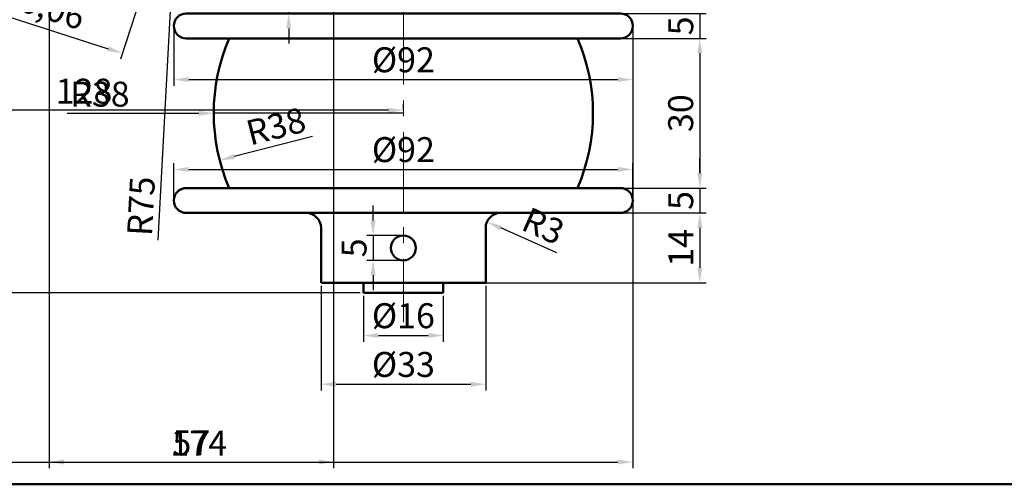
# Model space of a CAD drawing. Units: millimetres. Extents: x 98 to 674, y 38 to 476.
# Tile 2 of 7: x 200 to 398, y 38 to 131. Entities that reach past the tile are written whole.
import ezdxf

# ---------------------------------------------------------------- set-up
doc = ezdxf.new("R2010")
doc.units = ezdxf.units.MM
doc.header["$LTSCALE"] = 0.5
doc.linetypes.add('CENTER', pattern=[50.8, 31.75, -6.35, 6.35, -6.35])
for name, color, linetype, lineweight in [('M-CNTR', 1, 'CENTER', 18), ('M-DIMS', 2, 'Continuous', 25), ('M-OUTL', 7, 'Continuous', 50), ('M-TTLB', 7, 'Continuous', 50)]:
    doc.layers.add(name, color=color, linetype=linetype, lineweight=lineweight)
doc.styles.get("Standard").update_dxf_attribs({"font": 'arial.ttf'})
doc.dimstyles.new('ISO-25', dxfattribs={"dimtxt": 5, "dimasz": 3, "dimexe": 1.25, "dimexo": 0.625, "dimtad": 1, "dimtxsty": 'Standard', "dimcen": 2.5, "dimadec": 0, "dimazin": 0, "dimtfac": 1, "dimtmove": 0, "dimatfit": 3, "dimfxl": 1, "dimarcsym": 0})

# ---------------------------------------------------------------- blocks, each defined once
blk = doc.blocks.new('*D38')
at = {"layer": 'Defpoints', "color": 0, "ltscale": 0.5, "transparency": 16777216}
for p in [(254.39, 138.69), (254.39, 132.69), (254.39, 132.69)]:
    blk.add_point(p, dxfattribs=at)
at = {"layer": 'M-DIMS', "color": 0, "lineweight": -2, "ltscale": 0.5, "transparency": 16777216}
for p, q in [((254.39, 141.69), (254.39, 144.69)), ((254.39, 138.69), (254.39, 132.69)), ((255.02, 138.69), (255.64, 138.69)), ((255.02, 132.69), (255.64, 132.69)), ((254.39, 129.69), (254.39, 126.69))]:
    blk.add_line(p, q, dxfattribs=at)
at = {"layer": 'M-DIMS', "color": 0, "ltscale": 0.5, "transparency": 16777216}
for points in [[(253.89, 141.69), (254.89, 141.69), (254.39, 138.69)], [(253.89, 129.69), (254.89, 129.69), (254.39, 132.69)]]:
    blk.add_solid(points, dxfattribs=at)
at = {"layer": 'M-DIMS', "color": 0, "ltscale": 0.5, "transparency": 16777216, "insert": (251.21, 135.69), "char_height": 5, "attachment_point": 5, "rotation": 90}
blk.add_mtext('6', dxfattribs=at)
blk = doc.blocks.new('*D39')
at = {"layer": 'Defpoints', "color": 0, "ltscale": 0.5, "transparency": 16777216}
for p in [(231.37, 130.19), (323.37, 130.19), (323.37, 119.43)]:
    blk.add_point(p, dxfattribs=at)
at = {"layer": 'M-DIMS', "color": 0, "lineweight": -2, "ltscale": 0.5, "transparency": 16777216}
for p, q in [((231.37, 129.56), (231.37, 118.18)), ((323.37, 129.56), (323.37, 118.18)), ((234.37, 119.43), (320.37, 119.43))]:
    blk.add_line(p, q, dxfattribs=at)
at = {"layer": 'M-DIMS', "color": 0, "ltscale": 0.5, "transparency": 16777216}
for points in [[(234.37, 119.93), (234.37, 118.93), (231.37, 119.43)], [(320.37, 119.93), (320.37, 118.93), (323.37, 119.43)]]:
    blk.add_solid(points, dxfattribs=at)
at = {"layer": 'M-DIMS', "color": 0, "ltscale": 0.5, "transparency": 16777216, "insert": (277.37, 122.75), "char_height": 5, "attachment_point": 5}
blk.add_mtext('%%C92', dxfattribs=at)
blk = doc.blocks.new('*D40')
at = {"layer": 'Defpoints', "color": 0, "ltscale": 0.5, "transparency": 16777216}
for p in [(277.37, 112.69), (240.56, 103.24)]:
    blk.add_point(p, dxfattribs=at)
at = {"layer": 'M-DIMS', "color": 0, "lineweight": -2, "ltscale": 0.5, "transparency": 16777216}
blk.add_line((259.16, 108.02), (243.46, 103.99), dxfattribs=at)
at = {"layer": 'M-DIMS', "color": 0, "ltscale": 0.5, "transparency": 16777216}
blk.add_solid([(243.34, 104.47), (243.59, 103.5), (240.56, 103.24)], dxfattribs=at)
at = {"layer": 'M-DIMS', "color": 0, "ltscale": 0.5, "transparency": 16777216, "insert": (251.98, 109.45), "char_height": 5, "attachment_point": 5, "rotation": 14.3875}
blk.add_mtext('R38', dxfattribs=at)
blk = doc.blocks.new('*D41')
at = {"layer": 'Defpoints', "color": 0, "ltscale": 0.5, "transparency": 16777216}
for p in [(323.37, 101.42), (231.37, 95.19), (323.37, 95.19)]:
    blk.add_point(p, dxfattribs=at)
at = {"layer": 'M-DIMS', "color": 0, "lineweight": -2, "ltscale": 0.5, "transparency": 16777216}
for p, q in [((231.37, 95.81), (231.37, 102.67)), ((323.37, 95.81), (323.37, 102.67)), ((234.37, 101.42), (320.37, 101.42))]:
    blk.add_line(p, q, dxfattribs=at)
at = {"layer": 'M-DIMS', "color": 0, "ltscale": 0.5, "transparency": 16777216}
for points in [[(234.37, 101.92), (234.37, 100.92), (231.37, 101.42)], [(320.37, 101.92), (320.37, 100.92), (323.37, 101.42)]]:
    blk.add_solid(points, dxfattribs=at)
at = {"layer": 'M-DIMS', "color": 0, "ltscale": 0.5, "transparency": 16777216, "insert": (277.37, 104.74), "char_height": 5, "attachment_point": 5}
blk.add_mtext('%%C92', dxfattribs=at)
blk = doc.blocks.new('*D42')
at = {"layer": 'Defpoints', "color": 0, "ltscale": 0.5, "transparency": 16777216}
for p in [(316.66, 132.69), (316.66, 127.69), (336.77, 127.69)]:
    blk.add_point(p, dxfattribs=at)
at = {"layer": 'M-DIMS', "color": 0, "lineweight": -2, "ltscale": 0.5, "transparency": 16777216}
for p, q in [((336.77, 135.69), (336.77, 138.69)), ((317.29, 132.69), (338.02, 132.69)), ((336.77, 132.69), (336.77, 127.69)), ((317.29, 127.69), (338.02, 127.69)), ((336.77, 124.69), (336.77, 121.69))]:
    blk.add_line(p, q, dxfattribs=at)
at = {"layer": 'M-DIMS', "color": 0, "ltscale": 0.5, "transparency": 16777216}
for points in [[(336.27, 135.69), (337.27, 135.69), (336.77, 132.69)], [(336.27, 124.69), (337.27, 124.69), (336.77, 127.69)]]:
    blk.add_solid(points, dxfattribs=at)
at = {"layer": 'M-DIMS', "color": 0, "ltscale": 0.5, "transparency": 16777216, "insert": (333.6, 130.19), "char_height": 5, "attachment_point": 5, "rotation": 90}
blk.add_mtext('5', dxfattribs=at)
blk = doc.blocks.new('*D43')
at = {"layer": 'Defpoints', "color": 0, "ltscale": 0.5, "transparency": 16777216}
for p in [(316.66, 127.69), (316.66, 97.69), (336.77, 97.69)]:
    blk.add_point(p, dxfattribs=at)
at = {"layer": 'M-DIMS', "color": 0, "lineweight": -2, "ltscale": 0.5, "transparency": 16777216}
for p, q in [((317.29, 127.69), (338.02, 127.69)), ((336.77, 124.69), (336.77, 100.69)), ((317.29, 97.69), (338.02, 97.69))]:
    blk.add_line(p, q, dxfattribs=at)
at = {"layer": 'M-DIMS', "color": 0, "ltscale": 0.5, "transparency": 16777216}
for points in [[(336.27, 124.69), (337.27, 124.69), (336.77, 127.69)], [(336.27, 100.69), (337.27, 100.69), (336.77, 97.69)]]:
    blk.add_solid(points, dxfattribs=at)
at = {"layer": 'M-DIMS', "color": 0, "ltscale": 0.5, "transparency": 16777216, "insert": (333.59, 112.69), "char_height": 5, "attachment_point": 5, "rotation": 90}
blk.add_mtext('30', dxfattribs=at)
blk = doc.blocks.new('*D44')
at = {"layer": 'Defpoints', "color": 0, "ltscale": 0.5, "transparency": 16777216}
for p in [(316.66, 97.69), (316.66, 92.69), (336.77, 92.69)]:
    blk.add_point(p, dxfattribs=at)
at = {"layer": 'M-DIMS', "color": 0, "lineweight": -2, "ltscale": 0.5, "transparency": 16777216}
for p, q in [((336.77, 100.69), (336.77, 103.69)), ((317.29, 97.69), (338.02, 97.69)), ((336.77, 97.69), (336.77, 92.69)), ((317.29, 92.69), (338.02, 92.69)), ((336.77, 89.69), (336.77, 86.69))]:
    blk.add_line(p, q, dxfattribs=at)
at = {"layer": 'M-DIMS', "color": 0, "ltscale": 0.5, "transparency": 16777216}
for points in [[(336.27, 100.69), (337.27, 100.69), (336.77, 97.69)], [(336.27, 89.69), (337.27, 89.69), (336.77, 92.69)]]:
    blk.add_solid(points, dxfattribs=at)
at = {"layer": 'M-DIMS', "color": 0, "ltscale": 0.5, "transparency": 16777216, "insert": (333.6, 95.19), "char_height": 5, "attachment_point": 5, "rotation": 90}
blk.add_mtext('5', dxfattribs=at)
blk = doc.blocks.new('*D45')
at = {"layer": 'Defpoints', "color": 0, "ltscale": 0.5, "transparency": 16777216}
for p in [(288.74, 92.69), (288.74, 78.69), (336.77, 78.69)]:
    blk.add_point(p, dxfattribs=at)
at = {"layer": 'M-DIMS', "color": 0, "lineweight": -2, "ltscale": 0.5, "transparency": 16777216}
for p, q in [((289.36, 92.69), (338.02, 92.69)), ((336.77, 89.69), (336.77, 81.69)), ((289.36, 78.69), (338.02, 78.69))]:
    blk.add_line(p, q, dxfattribs=at)
at = {"layer": 'M-DIMS', "color": 0, "ltscale": 0.5, "transparency": 16777216}
for points in [[(336.27, 89.69), (337.27, 89.69), (336.77, 92.69)], [(336.27, 81.69), (337.27, 81.69), (336.77, 78.69)]]:
    blk.add_solid(points, dxfattribs=at)
at = {"layer": 'M-DIMS', "color": 0, "ltscale": 0.5, "transparency": 16777216, "insert": (333.64, 85.69), "char_height": 5, "attachment_point": 5, "rotation": 90}
blk.add_mtext('14', dxfattribs=at)
blk = doc.blocks.new('*D46')
at = {"layer": 'Defpoints', "color": 0, "ltscale": 0.5, "transparency": 16777216}
for p in [(277.37, 88.19), (271.3, 83.19), (277.37, 83.19)]:
    blk.add_point(p, dxfattribs=at)
at = {"layer": 'M-DIMS', "color": 0, "lineweight": -2, "ltscale": 0.5, "transparency": 16777216}
for p, q in [((271.3, 91.19), (271.3, 94.19)), ((276.74, 88.19), (270.05, 88.19)), ((271.3, 88.19), (271.3, 83.19)), ((276.74, 83.19), (270.05, 83.19)), ((271.3, 80.19), (271.3, 77.19))]:
    blk.add_line(p, q, dxfattribs=at)
at = {"layer": 'M-DIMS', "color": 0, "ltscale": 0.5, "transparency": 16777216}
for points in [[(270.8, 91.19), (271.8, 91.19), (271.3, 88.19)], [(270.8, 80.19), (271.8, 80.19), (271.3, 83.19)]]:
    blk.add_solid(points, dxfattribs=at)
at = {"layer": 'M-DIMS', "color": 0, "ltscale": 0.5, "transparency": 16777216, "insert": (268.13, 85.69), "char_height": 5, "attachment_point": 5, "rotation": 90}
blk.add_mtext('5', dxfattribs=at)
blk = doc.blocks.new('*D47')
at = {"layer": 'Defpoints', "color": 0, "ltscale": 0.5, "transparency": 16777216}
for p in [(269.37, 76.69), (285.37, 76.69), (285.37, 68.12)]:
    blk.add_point(p, dxfattribs=at)
at = {"layer": 'M-DIMS', "color": 0, "lineweight": -2, "ltscale": 0.5, "transparency": 16777216}
for p, q in [((269.37, 76.06), (269.37, 66.87)), ((285.37, 76.06), (285.37, 66.87)), ((272.37, 68.12), (282.37, 68.12))]:
    blk.add_line(p, q, dxfattribs=at)
at = {"layer": 'M-DIMS', "color": 0, "ltscale": 0.5, "transparency": 16777216}
for points in [[(272.37, 68.62), (272.37, 67.62), (269.37, 68.12)], [(282.37, 68.62), (282.37, 67.62), (285.37, 68.12)]]:
    blk.add_solid(points, dxfattribs=at)
at = {"layer": 'M-DIMS', "color": 0, "ltscale": 0.5, "transparency": 16777216, "insert": (277.37, 71.44), "char_height": 5, "attachment_point": 5}
blk.add_mtext('%%C16', dxfattribs=at)
blk = doc.blocks.new('*D48')
at = {"layer": 'Defpoints', "color": 0, "ltscale": 0.5, "transparency": 16777216}
for p in [(260.87, 78.69), (293.87, 78.69), (293.87, 58.35)]:
    blk.add_point(p, dxfattribs=at)
at = {"layer": 'M-DIMS', "color": 0, "lineweight": -2, "ltscale": 0.5, "transparency": 16777216}
for p, q in [((260.87, 78.06), (260.87, 57.1)), ((293.87, 78.06), (293.87, 57.1)), ((263.87, 58.35), (290.87, 58.35))]:
    blk.add_line(p, q, dxfattribs=at)
at = {"layer": 'M-DIMS', "color": 0, "ltscale": 0.5, "transparency": 16777216}
for points in [[(263.87, 58.85), (263.87, 57.85), (260.87, 58.35)], [(290.87, 58.85), (290.87, 57.85), (293.87, 58.35)]]:
    blk.add_solid(points, dxfattribs=at)
at = {"layer": 'M-DIMS', "color": 0, "ltscale": 0.5, "transparency": 16777216, "insert": (277.37, 61.67), "char_height": 5, "attachment_point": 5}
blk.add_mtext('%%C33', dxfattribs=at)
blk = doc.blocks.new('*D49')
at = {"layer": 'Defpoints', "color": 0, "ltscale": 0.5, "transparency": 16777216}
for p in [(294.12, 90.9), (296.87, 89.69)]:
    blk.add_point(p, dxfattribs=at)
at = {"layer": 'M-DIMS', "color": 0, "lineweight": -2, "ltscale": 0.5, "transparency": 16777216}
blk.add_line((308.12, 84.7), (296.87, 89.69), dxfattribs=at)
at = {"layer": 'M-DIMS', "color": 0, "ltscale": 0.5, "transparency": 16777216}
blk.add_solid([(297.07, 90.14), (296.66, 89.23), (294.12, 90.9)], dxfattribs=at)
at = {"layer": 'M-DIMS', "color": 0, "ltscale": 0.5, "transparency": 16777216, "insert": (305.15, 89.5), "char_height": 5, "attachment_point": 5, "rotation": 336.1343}
blk.add_mtext('R3', dxfattribs=at)
blk = doc.blocks.new('*D50')
at = {"layer": 'Defpoints', "color": 0, "ltscale": 0.5, "transparency": 16777216}
for p in [(149.37, 153.69), (149.37, 113.28), (277.37, 112.69)]:
    blk.add_point(p, dxfattribs=at)
at = {"layer": 'M-DIMS', "color": 0, "lineweight": -2, "ltscale": 0.5, "transparency": 16777216}
for p, q in [((149.37, 153.06), (149.37, 112.03)), ((277.37, 113.31), (277.37, 114.53)), ((274.37, 113.28), (152.37, 113.28))]:
    blk.add_line(p, q, dxfattribs=at)
at = {"layer": 'M-DIMS', "color": 0, "ltscale": 0.5, "transparency": 16777216}
for points in [[(152.37, 113.78), (152.37, 112.78), (149.37, 113.28)], [(274.37, 113.78), (274.37, 112.78), (277.37, 113.28)]]:
    blk.add_solid(points, dxfattribs=at)
at = {"layer": 'M-DIMS', "color": 0, "ltscale": 0.5, "transparency": 16777216, "insert": (213.37, 116.46), "char_height": 5, "attachment_point": 5}
blk.add_mtext('128', dxfattribs=at)
blk = doc.blocks.new('*D53')
at = {"layer": 'Defpoints', "color": 0, "ltscale": 0.5, "transparency": 16777216}
for p in [(192.69, 154.23), (227.02, 143.17), (221.06, 124.69)]:
    blk.add_point(p, dxfattribs=at)
at = {"layer": 'M-DIMS', "color": 0, "lineweight": -2, "ltscale": 0.5, "transparency": 16777216}
for p, q in [((192.5, 153.64), (186.35, 134.56)), ((226.82, 142.58), (220.68, 123.5)), ((189.59, 134.83), (218.21, 125.61))]:
    blk.add_line(p, q, dxfattribs=at)
at = {"layer": 'M-DIMS', "color": 0, "ltscale": 0.5, "transparency": 16777216}
for points in [[(189.75, 135.31), (189.44, 134.36), (186.74, 135.75)], [(218.36, 126.09), (218.05, 125.14), (221.06, 124.69)]]:
    blk.add_solid(points, dxfattribs=at)
at = {"layer": 'M-DIMS', "color": 0, "ltscale": 0.5, "transparency": 16777216, "insert": (205.01, 133.68), "char_height": 5, "attachment_point": 5, "rotation": 342.137}
blk.add_mtext('36,06', dxfattribs=at)
blk = doc.blocks.new('*D68')
at = {"layer": 'Defpoints', "color": 0, "ltscale": 0.5, "transparency": 16777216}
for p in [(263.37, 325.69), (206.37, 226.96), (263.37, 42.76)]:
    blk.add_point(p, dxfattribs=at)
at = {"layer": 'M-DIMS', "color": 0, "lineweight": -2, "ltscale": 0.5, "transparency": 16777216}
for p, q in [((263.37, 325.06), (263.37, 41.51)), ((206.37, 226.33), (206.37, 41.51)), ((209.37, 42.76), (260.37, 42.76))]:
    blk.add_line(p, q, dxfattribs=at)
at = {"layer": 'M-DIMS', "color": 0, "ltscale": 0.5, "transparency": 16777216}
for points in [[(209.37, 43.26), (209.37, 42.26), (206.37, 42.76)], [(260.37, 43.26), (260.37, 42.26), (263.37, 42.76)]]:
    blk.add_solid(points, dxfattribs=at)
at = {"layer": 'M-DIMS', "color": 0, "ltscale": 0.5, "transparency": 16777216, "insert": (234.87, 45.93), "char_height": 5, "attachment_point": 5}
blk.add_mtext('57', dxfattribs=at)
blk = doc.blocks.new('*D71')
at = {"layer": 'Defpoints', "color": 0, "ltscale": 0.5, "transparency": 16777216}
for p in [(269.37, 413.69), (121.37, 76.69), (269.37, 76.69)]:
    blk.add_point(p, dxfattribs=at)
at = {"layer": 'M-DIMS', "color": 0, "lineweight": -2, "ltscale": 0.5, "transparency": 16777216}
for p, q in [((268.74, 413.69), (120.12, 413.69)), ((121.37, 410.69), (121.37, 79.69)), ((268.74, 76.69), (120.12, 76.69))]:
    blk.add_line(p, q, dxfattribs=at)
at = {"layer": 'M-DIMS', "color": 0, "ltscale": 0.5, "transparency": 16777216}
for points in [[(120.87, 410.69), (121.87, 410.69), (121.37, 413.69)], [(120.87, 79.69), (121.87, 79.69), (121.37, 76.69)]]:
    blk.add_solid(points, dxfattribs=at)
at = {"layer": 'M-DIMS', "color": 0, "ltscale": 0.5, "transparency": 16777216, "insert": (118.19, 245.19), "char_height": 5, "attachment_point": 5, "rotation": 90}
blk.add_mtext('337', dxfattribs=at)
blk = doc.blocks.new('*D72')
at = {"layer": 'Defpoints', "color": 0, "ltscale": 0.5, "transparency": 16777216}
for p in [(149.37, 196.69), (323.37, 130.19), (323.37, 42.76)]:
    blk.add_point(p, dxfattribs=at)
at = {"layer": 'M-DIMS', "color": 0, "lineweight": -2, "ltscale": 0.5, "transparency": 16777216}
for p, q in [((149.37, 196.06), (149.37, 41.51)), ((323.37, 129.56), (323.37, 41.51)), ((152.37, 42.76), (320.37, 42.76))]:
    blk.add_line(p, q, dxfattribs=at)
at = {"layer": 'M-DIMS', "color": 0, "ltscale": 0.5, "transparency": 16777216}
for points in [[(152.37, 43.26), (152.37, 42.26), (149.37, 42.76)], [(320.37, 43.26), (320.37, 42.26), (323.37, 42.76)]]:
    blk.add_solid(points, dxfattribs=at)
at = {"layer": 'M-DIMS', "color": 0, "ltscale": 0.5, "transparency": 16777216, "insert": (236.37, 45.9), "char_height": 5, "attachment_point": 5}
blk.add_mtext('174', dxfattribs=at)
blk = doc.blocks.new('*D76')
at = {"layer": 'Defpoints', "color": 0, "ltscale": 0.5, "transparency": 16777216}
for p in [(234.98, 213.69), (230.99, 138.79)]:
    blk.add_point(p, dxfattribs=at)
at = {"layer": 'M-DIMS', "color": 0, "lineweight": -2, "ltscale": 0.5, "transparency": 16777216}
for p, q in [((234.98, 213.69), (230.99, 138.79)), ((228.25, 87.25), (230.84, 135.8))]:
    blk.add_line(p, q, dxfattribs=at)
at = {"layer": 'M-DIMS', "color": 0, "ltscale": 0.5, "transparency": 16777216}
blk.add_solid([(230.34, 135.82), (231.33, 135.77), (230.99, 138.79)], dxfattribs=at)
at = {"layer": 'M-DIMS', "color": 0, "ltscale": 0.5, "transparency": 16777216, "insert": (225.44, 94.02), "char_height": 5, "attachment_point": 5, "rotation": 86.9505}
blk.add_mtext('R75', dxfattribs=at)
blk = doc.blocks.new('*D77')
at = {"layer": 'Defpoints', "color": 0, "ltscale": 0.5, "transparency": 16777216}
for p in [(239.37, 112.68), (277.37, 112.69)]:
    blk.add_point(p, dxfattribs=at)
at = {"layer": 'M-DIMS', "color": 0, "lineweight": -2, "ltscale": 0.5, "transparency": 16777216}
for p, q in [((209.96, 112.68), (236.37, 112.68)), ((277.37, 112.69), (239.37, 112.68))]:
    blk.add_line(p, q, dxfattribs=at)
at = {"layer": 'M-DIMS', "color": 0, "ltscale": 0.5, "transparency": 16777216}
blk.add_solid([(236.37, 113.18), (236.37, 112.18), (239.37, 112.68)], dxfattribs=at)
at = {"layer": 'M-DIMS', "color": 0, "ltscale": 0.5, "transparency": 16777216, "insert": (216.56, 115.86), "char_height": 5, "attachment_point": 5, "rotation": 0.0007}
blk.add_mtext('R38', dxfattribs=at)

msp = doc.modelspace()

# ---------------------------------------------------------------- linework, layer by layer
at = {"layer": 'M-CNTR'}
msp.add_line((277.365, 413.6855), (277.365, 70.7639), dxfattribs=at)
at = {"layer": 'M-OUTL'}
for p, q in [((296.865, 92.6855), (320.865, 92.6855)), ((260.865, 78.6855), (260.865, 89.6855)), ((293.865, 89.6855), (293.865, 78.6855)), ((293.865, 78.6855), (260.865, 78.6855)), ((269.365, 78.6855), (285.365, 78.6855)), ((269.365, 76.6855), (269.365, 78.6855)), ((285.365, 78.6855), (285.365, 76.6855)), ((285.365, 76.6855), (269.365, 76.6855))]:
    msp.add_line(p, q, dxfattribs=at)
for points in [[(320.865, 132.6855), (233.865, 132.6855, 1), (233.865, 127.6855), (320.865, 127.6855, 1)], [(320.865, 97.6855), (233.865, 97.6855, 1), (233.865, 92.6855), (320.865, 92.6855, 1)]]:
    msp.add_lwpolyline(points, format="xyb", close=True, dxfattribs=at)
msp.add_circle((277.365, 85.6855), 2.5, dxfattribs=at)
for centre, radius, start, end in [((277.365, 112.6855), 38, 156.750437, 203.249563), ((277.365, 112.6855), 38, 336.750437, 23.249563), ((257.865, 89.6855), 3, 0, 90), ((296.865, 89.6855), 3, 90, 180)]:
    msp.add_arc(centre, radius, start, end, dxfattribs=at)
at = {"layer": 'M-TTLB', "ltscale": 0.5}
msp.add_lwpolyline([(98.2162, 475.6271), (666.7064, 475.6271), (666.7064, 38.2873), (98.2162, 38.2873)], close=True, dxfattribs=at)

# ---------------------------------------------------------------- dimensions: what is measured, and where the dimension line sits
at = {"layer": 'M-DIMS', "ltscale": 0.5}
for base, p1, p2, override, picture, middle in [((121.365, 76.6855), (269.365, 413.6855), (269.365, 76.6855), {"dimdec": 0, "dimlfac": 1, "dimrnd": 0, "dimzin": 0, "dimdsep": 46, "dimlunit": 2}, '*D71', (118.1855, 245.1855)), ((254.3923, 132.6855), (254.3923, 138.6855), (254.3923, 132.6855), {"dimclrd": 0, "dimclre": 0, "dimclrt": 0}, '*D38', (251.2145, 135.6855)), ((336.7704, 127.6855), (316.6618, 132.6855), (316.6618, 127.6855), {"dimclrd": 0, "dimclre": 0, "dimclrt": 0}, '*D42', (333.6027, 130.1855)), ((336.7704, 97.6855), (316.6618, 127.6855), (316.6618, 97.6855), {"dimclrd": 0, "dimclre": 0, "dimclrt": 0}, '*D43', (333.5908, 112.6855)), ((336.7704, 92.6855), (316.6618, 97.6855), (316.6618, 92.6855), {"dimclrd": 0, "dimclre": 0, "dimclrt": 0}, '*D44', (333.6027, 95.1855)), ((271.2997, 83.1855), (277.365, 88.1855), (277.365, 83.1855), {"dimclrd": 0, "dimclre": 0, "dimclrt": 0}, '*D46', (268.132, 85.6855)), ((336.7704, 78.6855), (288.7376, 92.6855), (288.7376, 78.6855), {"dimclrd": 0, "dimclre": 0, "dimclrt": 0}, '*D45', (333.6351, 85.6855))]:
    dim = msp.add_linear_dim(base=base, p1=p1, p2=p2, angle=90, dimstyle='ISO-25', override=override, dxfattribs=at)
    dim.commit()
    dim.dimension.update_dxf_attribs({"geometry": picture, "text_midpoint": middle})
for base, p1, p2, override, picture, middle in [((263.365, 42.7639), (206.365, 226.9586), (263.365, 325.6855), {"dimdec": 0, "dimlfac": 1, "dimrnd": 0, "dimzin": 0, "dimdsep": 46, "dimlunit": 2}, '*D68', (234.865, 45.9316)), ((323.365, 42.7639), (149.365, 196.6855), (323.365, 130.1855), {"dimdec": 0, "dimlfac": 1, "dimrnd": 0, "dimzin": 0, "dimdsep": 46, "dimlunit": 2}, '*D72', (236.365, 45.8992)), ((149.365, 113.2817), (277.365, 112.6855), (149.365, 153.6855), {"dimclrd": 0, "dimclre": 0, "dimclrt": 0}, '*D50', (213.365, 116.4596))]:
    dim = msp.add_linear_dim(base=base, p1=p1, p2=p2, dimstyle='ISO-25', override=override, dxfattribs=at)
    dim.commit()
    dim.dimension.update_dxf_attribs({"geometry": picture, "text_midpoint": middle})
for center, mpoint, override, picture, middle in [((234.9849, 213.6855), (230.995, 138.7917), {"dimdec": 0, "dimlfac": 1, "dimrnd": 0, "dimzin": 0, "dimdsep": 46, "dimlunit": 2}, '*D76', (228.601, 93.8554)), ((277.365, 112.6855), (239.365, 112.685), {"dimdec": 0, "dimlfac": 1, "dimrnd": 0, "dimzin": 0, "dimdsep": 46, "dimlunit": 2}, '*D77', (216.565, 112.6847)), ((277.365, 112.6855), (240.5568, 103.2433), {"dimclrd": 0, "dimclre": 0, "dimclrt": 0}, '*D40', (252.7654, 106.3751)), ((296.865, 89.6855), (294.1215, 90.8993), {"dimclrd": 0, "dimclre": 0, "dimclrt": 0}, '*D49', (303.8668, 86.5878))]:
    dim = msp.add_radius_dim(center=center, mpoint=mpoint, dimstyle='ISO-25', override=override, dxfattribs=at)
    dim.commit()
    dim.dimension.update_dxf_attribs({"geometry": picture, "text_midpoint": middle, "dimtype": 164})
dim = msp.add_aligned_dim(p1=(192.6933, 154.232), p2=(227.0163, 143.1705), distance=-19.4157, dimstyle='ISO-25', override={"dimclrd": 0, "dimclre": 0, "dimclrt": 0}, dxfattribs=at)
dim.commit()
dim.dimension.update_dxf_attribs({"geometry": '*D53', "text_midpoint": (205.0126, 133.6763)})
for base, p1, p2, picture, middle in [((323.365, 119.4303), (231.365, 130.1855), (323.365, 130.1855), '*D39', (277.365, 122.748)), ((323.365, 101.4245), (231.365, 95.1855), (323.365, 95.1855), '*D41', (277.365, 104.7422)), ((293.865, 58.353), (260.865, 78.6855), (293.865, 78.6855), '*D48', (277.365, 61.6707)), ((285.365, 68.1236), (269.365, 76.6855), (285.365, 76.6855), '*D47', (277.365, 71.4413))]:
    dim = msp.add_linear_dim(base=base, p1=p1, p2=p2, text='%%C<>', dimstyle='ISO-25', override={"dimclrd": 0, "dimclre": 0, "dimclrt": 0}, dxfattribs=at)
    dim.commit()
    dim.dimension.update_dxf_attribs({"geometry": picture, "text_midpoint": middle})

doc.saveas('drawing.dxf')
